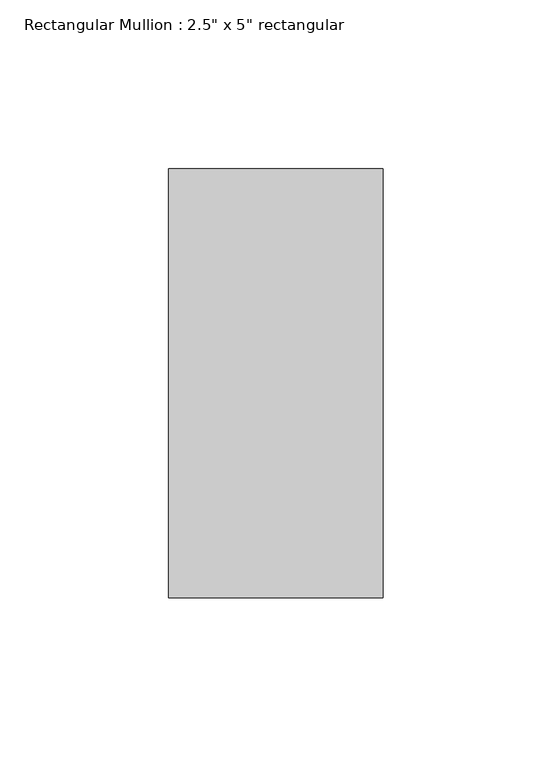
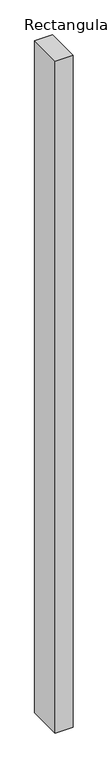
"""IFC4 building model written with IfcOpenShell, lengths in millimetres: member geometry."""

from ifc_helpers import new_model, si_unit, frame, origin, place, context, project, spatial, polyline, outline, extrude, source, transform, mapped, element, save


def member_2b3b556d(model_context):
    return source(origin(), model_context, "Body", "SweptSolid", [
        extrude(outline(polyline([(0.0, 63.5), (0.0, -63.5), (-63.5, -63.5), (-63.5, 63.5), (0.0, 63.5)])), frame((0.0, 0.0, -2540.0), z_axis=(0.0, 0.0, 1.0), x_axis=(1.0, 0.0, 0.0)), (0.0, 0.0, 1.0), 2540.0),
    ])


if __name__ == "__main__":
    model = new_model("IFC4")
    model_context = context("Model", 3, world=origin())
    ifc_project = project(units=[si_unit("LENGTHUNIT", "METRE", prefix="MILLI")], contexts=[model_context])
    site = spatial("IfcSite", under=ifc_project)
    building = spatial("IfcBuilding", under=site)
    placement = place(None, origin())
    member_shape = member_2b3b556d(model_context)
    element("IfcMember", 1, ObjectType="Rectangular Mullion : 2.5\" x 5\" rectangular", at=placement, inside=building, context=model_context, shape_type="MappedRepresentation", body=[
        mapped(member_shape, transform((0.0, 0.0, 0.0), x_axis=(1.0, 0.0, 0.0), y_axis=(0.0, 1.0, 0.0), z_axis=(0.0, 0.0, 1.0))),
    ])
    save(model, "model.ifc")

# Revit data of these elements
# Type "Rectangular Mullion : 2.5\" x 5\" rectangular"
#   built-in parameter 1007304 = 0.416667 (stored number, unit not read)
#   built-in parameter 1007301 = 0.104167 (stored number, unit not read)
#   built-in parameter 1007300 = 0.104167 (stored number, unit not read)
# Element 1 (IfcMember, "Rectangular Mullion : 2.5\" x 5\" rectangular")
#   Materials on its faces: "Aluminum"
# Materials
#   "Aluminum": class "Metal", colour RGB 247 247 247, transparency 0, Description = "Aluminum 6061", Cost = 0
